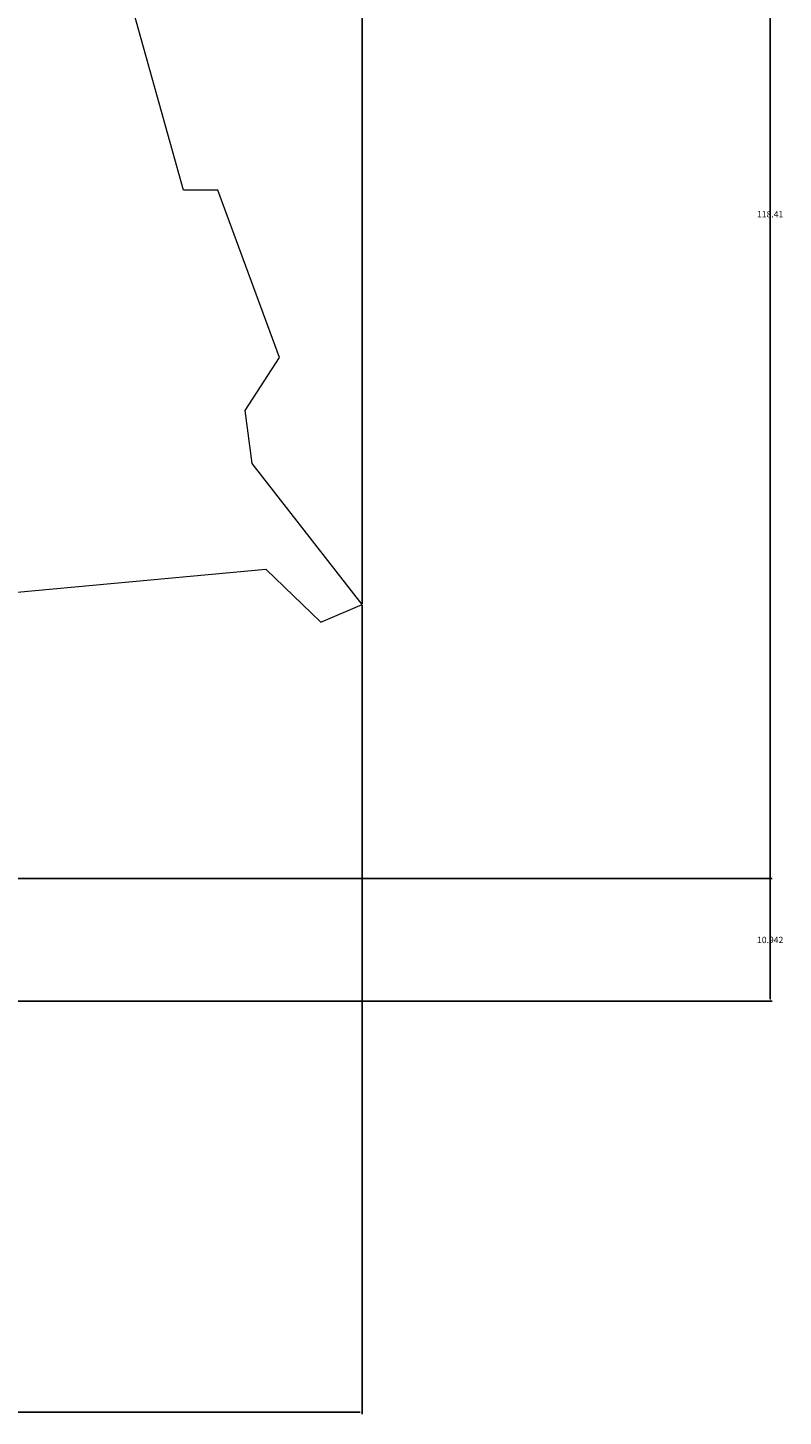
# Model space of a CAD drawing. Units: inches. Extents: x -26 to 776, y -22 to 650.
# Tile 52 of 62: x 709 to 776, y -22 to 102. Entities that reach past the tile are written whole.
import ezdxf

# ---------------------------------------------------------------- set-up
doc = ezdxf.new("R2010")
doc.units = ezdxf.units.IN
doc.header["$MEASUREMENT"] = 0
doc.layers.add('A-ANNO-DIMS', color=2, linetype='Continuous', lineweight=18)
doc.layers.add('L-PLNT-TREE', color=94, linetype='Continuous', lineweight=18)
doc.styles.get("Standard").update_dxf_attribs({"font": 'arial.ttf'})
doc.dimstyles.get("Standard").update_dxf_attribs({"dimtxt": 0.5625, "dimasz": 0.18, "dimexe": 0.18, "dimexo": 0.0625, "dimgap": 0.09, "dimtad": 0, "dimtih": 1, "dimtoh": 1, "dimdec": 4, "dimzin": 0, "dimdsep": 46, "dimlunit": 4, "dimtxsty": 'Standard', "dimcen": 0.09, "dimadec": 0, "dimazin": 0, "dimtfac": 1, "dimtdec": 4, "dimtofl": 0, "dimtmove": 0, "dimatfit": 3, "dimfxl": 1, "dimtolj": 1, "dimtzin": 0, "dimarcsym": 0})

# ---------------------------------------------------------------- blocks, each defined once
blk = doc.blocks.new('Tree - type 3 evergreen elevation')
blk.add_lwpolyline([(43.5651, 25.437), (61.6813, 27.0959), (65.132, 23.7781), (67.7201, 24.884), (60.8186, 33.7317), (60.3873, 37.0495), (62.544, 40.3674), (58.662, 50.874), (56.5053, 50.874), (52.1919, 66.3574)])
blk = doc.blocks.new('*D13')
at = {"layer": 'A-ANNO-DIMS', "color": 0, "lineweight": -2, "transparency": 16777216}
for p, q in [((738.75, 50.79), (738.75, -21.31)), ((11.11, 15.42), (11.11, -21.31)), ((11.29, -21.13), (373.89, -21.13)), ((738.57, -21.13), (375.97, -21.13))]:
    blk.add_line(p, q, dxfattribs=at)
at = {"layer": 'A-ANNO-DIMS', "color": 0, "transparency": 16777216}
for points in [[(11.29, -21.1), (11.29, -21.16), (11.11, -21.13)], [(738.57, -21.1), (738.57, -21.16), (738.75, -21.13)]]:
    blk.add_solid(points, dxfattribs=at)
at = {"layer": 'Defpoints', "color": 0, "transparency": 16777216}
for p in [(738.75, 50.85), (11.11, 15.48), (738.75, -21.13)]:
    blk.add_point(p, dxfattribs=at)
at = {"layer": 'A-ANNO-DIMS', "color": 0, "transparency": 16777216, "insert": (374.93, -21.13), "char_height": 0.562, "attachment_point": 5}
blk.add_mtext('\\A1;727.6', dxfattribs=at)
blk = doc.blocks.new('*D20')
at = {"layer": 'A-ANNO-DIMS', "color": 0, "lineweight": -2, "transparency": 16777216}
for p, q in [((425.81, 455.47), (775.34, 455.47)), ((775.16, 455.29), (775.16, 235.85)), ((775.16, 15.66), (775.16, 235.1)), ((425.81, 15.48), (775.34, 15.48))]:
    blk.add_line(p, q, dxfattribs=at)
at = {"layer": 'A-ANNO-DIMS', "color": 0, "transparency": 16777216}
for points in [[(775.13, 455.29), (775.19, 455.29), (775.16, 455.47)], [(775.13, 15.66), (775.19, 15.66), (775.16, 15.48)]]:
    blk.add_solid(points, dxfattribs=at)
at = {"layer": 'Defpoints', "color": 0, "transparency": 16777216}
for p in [(425.74, 455.47), (775.16, 455.47), (425.74, 15.48)]:
    blk.add_point(p, dxfattribs=at)
at = {"layer": 'A-ANNO-DIMS', "color": 0, "transparency": 16777216, "insert": (775.16, 235.48), "char_height": 0.562, "attachment_point": 5}
blk.add_mtext('\\A1;440', dxfattribs=at)
blk = doc.blocks.new('*D30')
at = {"layer": 'A-ANNO-DIMS', "color": 0, "lineweight": -2, "transparency": 16777216}
for p, q in [((280.68, 144.84), (775.34, 144.84)), ((775.16, 144.66), (775.16, 86.01)), ((775.16, 26.6), (775.16, 85.25)), ((280.68, 26.42), (775.34, 26.42))]:
    blk.add_line(p, q, dxfattribs=at)
at = {"layer": 'A-ANNO-DIMS', "color": 0, "transparency": 16777216}
for points in [[(775.13, 144.66), (775.19, 144.66), (775.16, 144.84)], [(775.13, 26.6), (775.19, 26.6), (775.16, 26.42)]]:
    blk.add_solid(points, dxfattribs=at)
at = {"layer": 'Defpoints', "color": 0, "transparency": 16777216}
for p in [(280.62, 144.84), (775.16, 144.84), (280.62, 26.42)]:
    blk.add_point(p, dxfattribs=at)
at = {"layer": 'A-ANNO-DIMS', "color": 0, "transparency": 16777216, "insert": (775.16, 85.63), "char_height": 0.562, "attachment_point": 5}
blk.add_mtext('\\A1;118.41', dxfattribs=at)
blk = doc.blocks.new('*D38')
at = {"layer": 'A-ANNO-DIMS', "color": 0, "lineweight": -2, "transparency": 16777216}
for p, q in [((280.68, 26.42), (775.34, 26.42)), ((775.16, 26.24), (775.16, 21.33)), ((775.16, 15.66), (775.16, 20.58)), ((289.3, 15.48), (775.34, 15.48))]:
    blk.add_line(p, q, dxfattribs=at)
at = {"layer": 'A-ANNO-DIMS', "color": 0, "transparency": 16777216}
for points in [[(775.13, 26.24), (775.19, 26.24), (775.16, 26.42)], [(775.13, 15.66), (775.19, 15.66), (775.16, 15.48)]]:
    blk.add_solid(points, dxfattribs=at)
at = {"layer": 'Defpoints', "color": 0, "transparency": 16777216}
for p in [(280.62, 26.42), (775.16, 26.42), (289.24, 15.48)]:
    blk.add_point(p, dxfattribs=at)
at = {"layer": 'A-ANNO-DIMS', "color": 0, "transparency": 16777216, "insert": (775.16, 20.95), "char_height": 0.562, "attachment_point": 5}
blk.add_mtext('\\A1;10.942', dxfattribs=at)
blk = doc.blocks.new('*D45')
at = {"layer": 'A-ANNO-DIMS', "color": 0, "lineweight": -2, "transparency": 16777216}
for p, q in [((507.74, 408.64), (775.34, 408.64)), ((775.16, 408.46), (775.16, 212.44)), ((775.16, 15.66), (775.16, 211.68)), ((586, 15.48), (775.34, 15.48))]:
    blk.add_line(p, q, dxfattribs=at)
at = {"layer": 'A-ANNO-DIMS', "color": 0, "transparency": 16777216}
for points in [[(775.13, 408.46), (775.19, 408.46), (775.16, 408.64)], [(775.13, 15.66), (775.19, 15.66), (775.16, 15.48)]]:
    blk.add_solid(points, dxfattribs=at)
at = {"layer": 'Defpoints', "color": 0, "transparency": 16777216}
for p in [(507.68, 408.64), (775.16, 408.64), (585.94, 15.48)]:
    blk.add_point(p, dxfattribs=at)
at = {"layer": 'A-ANNO-DIMS', "color": 0, "transparency": 16777216, "insert": (775.16, 212.06), "char_height": 0.562, "attachment_point": 5}
blk.add_mtext('\\A1;393.16', dxfattribs=at)
blk = doc.blocks.new('*D46')
at = {"layer": 'A-ANNO-DIMS', "color": 0, "lineweight": -2, "transparency": 16777216}
for p, q in [((658.51, 219.03), (775.34, 219.03)), ((775.16, 218.85), (775.16, 117.63)), ((775.16, 15.66), (775.16, 116.88)), ((677.97, 15.48), (775.34, 15.48))]:
    blk.add_line(p, q, dxfattribs=at)
at = {"layer": 'A-ANNO-DIMS', "color": 0, "transparency": 16777216}
for points in [[(775.13, 218.85), (775.19, 218.85), (775.16, 219.03)], [(775.13, 15.66), (775.19, 15.66), (775.16, 15.48)]]:
    blk.add_solid(points, dxfattribs=at)
at = {"layer": 'Defpoints', "color": 0, "transparency": 16777216}
for p in [(658.44, 219.03), (775.16, 219.03), (677.9, 15.48)]:
    blk.add_point(p, dxfattribs=at)
at = {"layer": 'A-ANNO-DIMS', "color": 0, "transparency": 16777216, "insert": (775.16, 117.26), "char_height": 0.562, "attachment_point": 5}
blk.add_mtext('\\A1;203.55', dxfattribs=at)
blk = doc.blocks.new('*D48')
at = {"layer": 'A-ANNO-DIMS', "color": 0, "lineweight": -2, "transparency": 16777216}
for p, q in [((545.03, 67.41), (545.03, 649.86)), ((738.75, 50.91), (738.75, 649.86)), ((545.21, 649.68), (640.88, 649.68)), ((738.57, 649.68), (642.9, 649.68))]:
    blk.add_line(p, q, dxfattribs=at)
at = {"layer": 'A-ANNO-DIMS', "color": 0, "transparency": 16777216}
for points in [[(545.21, 649.71), (545.21, 649.65), (545.03, 649.68)], [(738.57, 649.71), (738.57, 649.65), (738.75, 649.68)]]:
    blk.add_solid(points, dxfattribs=at)
at = {"layer": 'Defpoints', "color": 0, "transparency": 16777216}
for p in [(738.75, 649.68), (545.03, 67.35), (738.75, 50.85)]:
    blk.add_point(p, dxfattribs=at)
at = {"layer": 'A-ANNO-DIMS', "color": 0, "transparency": 16777216, "insert": (641.89, 649.68), "char_height": 0.562, "attachment_point": 5}
blk.add_mtext('\\A1;193.7', dxfattribs=at)

msp = doc.modelspace()

# ---------------------------------------------------------------- block references
at = {"layer": 'L-PLNT-TREE', "xscale": 1.421226385586178, "yscale": 1.421226385586178, "zscale": 1.421226385586178}
msp.add_blockref('Tree - type 3 evergreen elevation', (642.5048, 15.4824), dxfattribs=at)

# ---------------------------------------------------------------- dimensions: what is measured, and where the dimension line sits
at = {"layer": 'A-ANNO-DIMS'}
for base, p1, picture, middle in [((738.7503, 649.6763), (545.0331, 67.3523), '*D48', (641.8917, 649.6763)), ((738.7503, -21.1349), (11.1074, 15.4824), '*D13', (374.9289, -21.1349))]:
    dim = msp.add_linear_dim(base=base, p1=p1, p2=(738.7503, 50.8482), dimstyle='Standard', override={"dimdec": 1, "dimlfac": 1, "dimrnd": 0, "dimzin": 0, "dimdsep": 46, "dimlunit": 2}, dxfattribs=at)
    dim.commit()
    dim.dimension.update_dxf_attribs({"geometry": picture, "text_midpoint": middle})
for base, p1, p2, override, picture, middle in [((775.1553, 455.4717), (425.7434, 15.4824), (425.7434, 455.4717), {"dimdec": 0, "dimlfac": 1, "dimrnd": 0, "dimzin": 0, "dimdsep": 46, "dimlunit": 2}, '*D20', (775.1553, 235.477)), ((775.1553, 408.6389), (585.9354, 15.4824), (507.6759, 408.6389), {"dimdec": 2, "dimlfac": 1, "dimrnd": 0, "dimzin": 0, "dimdsep": 46, "dimlunit": 2}, '*D45', (775.1553, 212.0606)), ((775.1553, 219.0324), (677.9037, 15.4824), (658.4435, 219.0324), {"dimdec": 2, "dimlfac": 1, "dimrnd": 0, "dimzin": 0, "dimdsep": 46, "dimlunit": 2}, '*D46', (775.1553, 117.2574)), ((775.1553, 144.8359), (280.6173, 26.4239), (280.6173, 144.8359), {"dimdec": 2, "dimlfac": 1, "dimrnd": 0, "dimzin": 0, "dimdsep": 46, "dimlunit": 2}, '*D30', (775.1553, 85.6299)), ((775.15535, 26.4239), (289.24236, 15.48237), (280.61732, 26.4239), {"dimdec": 3, "dimlfac": 1, "dimrnd": 0, "dimzin": 0, "dimdsep": 46, "dimlunit": 2}, '*D38', (775.15535, 20.95313))]:
    dim = msp.add_linear_dim(base=base, p1=p1, p2=p2, angle=90, dimstyle='Standard', override=override, dxfattribs=at)
    dim.commit()
    dim.dimension.update_dxf_attribs({"geometry": picture, "text_midpoint": middle})

doc.saveas('drawing.dxf')
